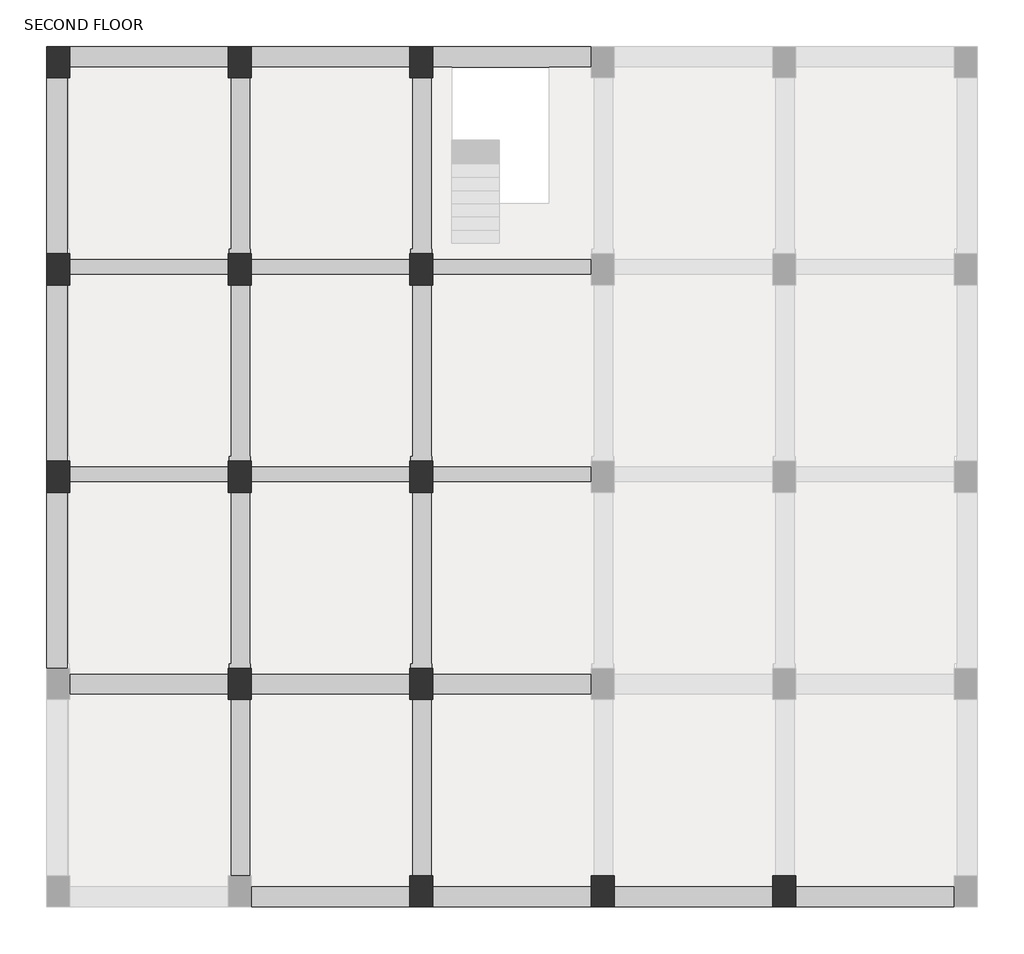
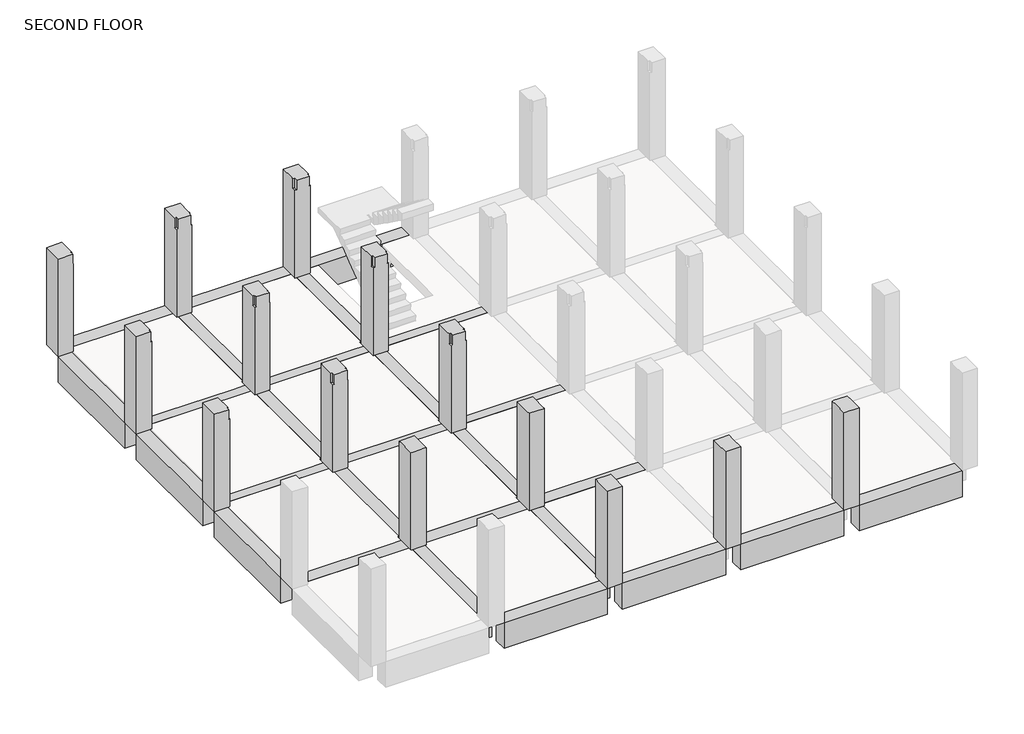
# One storey, part 2 of 3: 27 beams, 14 columns.
"""IFC4 building model written with IfcOpenShell, lengths in millimetres."""

from ifc_helpers import new_model, si_unit, frame, origin, place, context, project, spatial, polyline, outline, extrude, faceted_brep, element, save

model = new_model("IFC4")

# Units and contexts
model_context = context("Model", 3, world=origin())
ifc_project = project(units=[si_unit("LENGTHUNIT", "METRE", prefix="MILLI")], contexts=[model_context])

# Site, building, storey
site = spatial("IfcSite", under=ifc_project)
building = spatial("IfcBuilding", under=site)
storey = spatial("IfcBuildingStorey", under=building, Name="SECOND FLOOR", Elevation=6096.0)

# Beams
placement = place(None, origin())
element("IfcBeam", 1, ObjectType="M_Concrete-Rectangular Beam : 400 x 800mm", at=placement, inside=storey, context=model_context, shape_type="Brep", body=[
    faceted_brep([(4855.1115906, 3503.1212443, 6096.0), (4855.1115906, 3103.1212443, 6096.0), (7905.1115906, 3103.1212443, 6096.0), (7905.1115906, 3503.1212443, 6096.0), (4855.1115906, 3503.1212443, 5296.0), (4855.1115906, 3503.1212443, 5796.0), (7905.1115906, 3503.1212443, 5796.0), (7905.1115906, 3503.1212443, 5296.0), (4855.1115906, 3103.1212443, 5296.0), (7905.1115906, 3103.1212443, 5296.0)], [[[0, 1, 2, 3]], [[4, 5, 0, 3, 6, 7]], [[8, 4, 7, 9]], [[1, 8, 9, 2]], [[1, 0, 5, 4, 8]], [[3, 2, 9, 7, 6]]]),
])
element("IfcBeam", 2, ObjectType="M_Concrete-Rectangular Beam : 400 x 800mm", at=placement, inside=storey, context=model_context, shape_type="Brep", body=[
    faceted_brep([(1355.1115906, 3503.1212443, 6096.0), (1355.1115906, 3103.1212443, 6096.0), (4405.1115906, 3103.1212443, 6096.0), (4405.1115906, 3503.1212443, 6096.0), (1355.1115906, 3503.1212443, 5296.0), (1355.1115906, 3503.1212443, 5796.0), (4405.1115906, 3503.1212443, 5796.0), (4405.1115906, 3503.1212443, 5296.0), (1355.1115906, 3103.1212443, 5296.0), (4405.1115906, 3103.1212443, 5296.0)], [[[0, 1, 2, 3]], [[4, 5, 0, 3, 6, 7]], [[8, 4, 7, 9]], [[1, 8, 9, 2]], [[1, 0, 5, 4, 8]], [[3, 2, 9, 7, 6]]]),
])
element("IfcBeam", 3, ObjectType="M_Concrete-Rectangular Beam : 400 x 800mm", at=placement, inside=storey, context=model_context, shape_type="Brep", body=[
    faceted_brep([(-2144.8884094, 3503.1212443, 6096.0), (-2144.8884094, 3103.1212443, 6096.0), (905.1115906, 3103.1212443, 6096.0), (905.1115906, 3503.1212443, 6096.0), (-2144.8884094, 3503.1212443, 5296.0), (-2144.8884094, 3503.1212443, 5796.0), (905.1115906, 3503.1212443, 5796.0), (905.1115906, 3503.1212443, 5296.0), (-2144.8884094, 3103.1212443, 5296.0), (905.1115906, 3103.1212443, 5296.0)], [[[0, 1, 2, 3]], [[4, 5, 0, 3, 6, 7]], [[8, 4, 7, 9]], [[1, 8, 9, 2]], [[1, 0, 5, 4, 8]], [[3, 2, 9, 7, 6]]]),
])
element("IfcBeam", 4, ObjectType="M_Concrete-Rectangular Beam : 400 x 800mm", at=placement, inside=storey, context=model_context, shape_type="Brep", body=[
    faceted_brep([(-5644.8884094, 3503.1212443, 6096.0), (-5644.8884094, 3103.1212443, 6096.0), (-2594.8884094, 3103.1212443, 6096.0), (-2594.8884094, 3503.1212443, 6096.0), (-5644.8884094, 3503.1212443, 5296.0), (-5644.8884094, 3503.1212443, 5796.0), (-2594.8884094, 3503.1212443, 5796.0), (-2594.8884094, 3503.1212443, 5296.0), (-5644.8884094, 3103.1212443, 5296.0), (-2594.8884094, 3103.1212443, 5296.0)], [[[0, 1, 2, 3]], [[4, 5, 0, 3, 6, 7]], [[8, 4, 7, 9]], [[1, 8, 9, 2]], [[1, 0, 5, 4, 8]], [[3, 2, 9, 7, 6]]]),
])
element("IfcBeam", 5, ObjectType="M_Concrete-Rectangular Beam : 400 x 800mm", at=placement, inside=storey, context=model_context, shape_type="SweptSolid", body=[
    extrude(outline(polyline([(-9594.8884094, 11103.1212443), (-9194.8884094, 11103.1212443), (-9194.8884094, 7703.1212443), (-9594.8884094, 7703.1212443), (-9594.8884094, 11103.1212443)])), frame((0.0, 0.0, 5296.0), z_axis=(0.0, 0.0, 1.0), x_axis=(1.0, 0.0, 0.0)), (0.0, 0.0, 1.0), 800.0),
])
element("IfcBeam", 6, ObjectType="M_Concrete-Rectangular Beam : 400 x 800mm", at=placement, inside=storey, context=model_context, shape_type="SweptSolid", body=[
    extrude(outline(polyline([(-9594.8884094, 15103.1212443), (-9194.8884094, 15103.1212443), (-9194.8884094, 11703.1212443), (-9594.8884094, 11703.1212443), (-9594.8884094, 15103.1212443)])), frame((0.0, 0.0, 5296.0), z_axis=(0.0, 0.0, 1.0), x_axis=(1.0, 0.0, 0.0)), (0.0, 0.0, 1.0), 800.0),
])
element("IfcBeam", 7, ObjectType="M_Concrete-Rectangular Beam : 400 x 800mm", at=placement, inside=storey, context=model_context, shape_type="Brep", body=[
    faceted_brep([(-2594.8884094, 19303.1212443, 6096.0), (-2594.8884094, 19703.1212443, 6096.0), (-5644.8884094, 19703.1212443, 6096.0), (-5644.8884094, 19303.1212443, 6096.0), (-2594.8884094, 19303.1212443, 5296.0), (-2594.8884094, 19303.1212443, 5796.0), (-5644.8884094, 19303.1212443, 5796.0), (-5644.8884094, 19303.1212443, 5296.0), (-2594.8884094, 19703.1212443, 5296.0), (-5644.8884094, 19703.1212443, 5296.0)], [[[0, 1, 2, 3]], [[4, 5, 0, 3, 6, 7]], [[8, 4, 7, 9]], [[1, 8, 9, 2]], [[1, 0, 5, 4, 8]], [[3, 2, 9, 7, 6]]]),
])
element("IfcBeam", 8, ObjectType="M_Concrete-Rectangular Beam : 400 x 800mm", at=placement, inside=storey, context=model_context, shape_type="Brep", body=[
    faceted_brep([(-2144.8884094, 19703.1212443, 6096.0), (-2144.8884094, 19303.1212443, 6096.0), (-1784.8884094, 19303.1212443, 6096.0), (94.7115906, 19303.1212443, 6096.0), (905.1115906, 19303.1212443, 6096.0), (905.1115906, 19703.1212443, 6096.0), (-2144.8884094, 19303.1212443, 5796.0), (-2144.8884094, 19303.1212443, 5296.0), (905.1115906, 19303.1212443, 5296.0), (905.1115906, 19303.1212443, 5796.0), (-2144.8884094, 19703.1212443, 5296.0), (905.1115906, 19703.1212443, 5296.0)], [[[0, 1, 2, 3, 4, 5]], [[1, 6, 7, 8, 9, 4, 3, 2]], [[7, 10, 11, 8]], [[10, 0, 5, 11]], [[1, 0, 10, 7, 6]], [[5, 4, 9, 8, 11]]]),
])
element("IfcBeam", 9, ObjectType="M_Concrete-Rectangular Beam : 400 x 800mm", at=placement, inside=storey, context=model_context, shape_type="Brep", body=[
    faceted_brep([(-5669.8884094, 15703.1212443, 6096.0), (-5669.8884094, 15803.1212443, 6096.0), (-5669.8884094, 19103.1212443, 6096.0), (-6044.8884094, 19103.1212443, 6096.0), (-6044.8884094, 15803.1212443, 6096.0), (-6069.8884094, 15803.1212443, 6096.0), (-6069.8884094, 15703.1212443, 6096.0), (-6069.8884094, 19103.1212443, 5296.0), (-6069.8884094, 15703.1212443, 5296.0), (-6069.8884094, 15803.1212443, 5796.0), (-6069.8884094, 19103.1212443, 5796.0), (-5669.8884094, 19103.1212443, 5296.0), (-5669.8884094, 15703.1212443, 5296.0), (-6044.8884094, 19103.1212443, 5796.0), (-6044.8884094, 15803.1212443, 5796.0)], [[[0, 1, 2, 3, 4, 5, 6]], [[7, 8, 6, 5, 9, 10]], [[7, 11, 12, 8]], [[11, 2, 1, 0, 12]], [[11, 7, 10, 13, 3, 2]], [[0, 6, 8, 12]], [[9, 14, 13, 10]], [[14, 4, 3, 13]], [[4, 14, 9, 5]]]),
])
element("IfcBeam", 10, ObjectType="M_Concrete-Rectangular Beam : 400 x 800mm", at=placement, inside=storey, context=model_context, shape_type="Brep", body=[
    faceted_brep([(-5669.8884094, 11703.1212443, 6096.0), (-5669.8884094, 11803.1212443, 6096.0), (-5669.8884094, 15103.1212443, 6096.0), (-6044.8884094, 15103.1212443, 6096.0), (-6044.8884094, 11803.1212443, 6096.0), (-6069.8884094, 11803.1212443, 6096.0), (-6069.8884094, 11703.1212443, 6096.0), (-6069.8884094, 15103.1212443, 5296.0), (-6069.8884094, 11703.1212443, 5296.0), (-6069.8884094, 11803.1212443, 5796.0), (-6069.8884094, 15103.1212443, 5796.0), (-5669.8884094, 15103.1212443, 5296.0), (-5669.8884094, 11703.1212443, 5296.0), (-6044.8884094, 15103.1212443, 5796.0), (-6044.8884094, 11803.1212443, 5796.0)], [[[0, 1, 2, 3, 4, 5, 6]], [[7, 8, 6, 5, 9, 10]], [[7, 11, 12, 8]], [[11, 2, 1, 0, 12]], [[11, 7, 10, 13, 3, 2]], [[0, 6, 8, 12]], [[9, 14, 13, 10]], [[14, 4, 3, 13]], [[4, 14, 9, 5]]]),
])
element("IfcBeam", 11, ObjectType="M_Concrete-Rectangular Beam : 400 x 800mm", at=placement, inside=storey, context=model_context, shape_type="Brep", body=[
    faceted_brep([(-5669.8884094, 7703.1212443, 6096.0), (-5669.8884094, 7803.1212443, 6096.0), (-5669.8884094, 11103.1212443, 6096.0), (-6044.8884094, 11103.1212443, 6096.0), (-6044.8884094, 7803.1212443, 6096.0), (-6069.8884094, 7803.1212443, 6096.0), (-6069.8884094, 7703.1212443, 6096.0), (-6069.8884094, 11103.1212443, 5296.0), (-6069.8884094, 7703.1212443, 5296.0), (-6069.8884094, 7803.1212443, 5796.0), (-6069.8884094, 11103.1212443, 5796.0), (-5669.8884094, 11103.1212443, 5296.0), (-5669.8884094, 7703.1212443, 5296.0), (-6044.8884094, 11103.1212443, 5796.0), (-6044.8884094, 7803.1212443, 5796.0)], [[[0, 1, 2, 3, 4, 5, 6]], [[7, 8, 6, 5, 9, 10]], [[8, 7, 11, 12]], [[2, 1, 0, 12, 11]], [[2, 11, 7, 10, 13, 3]], [[0, 6, 8, 12]], [[9, 14, 13, 10]], [[14, 4, 3, 13]], [[4, 14, 9, 5]]]),
])
element("IfcBeam", 12, ObjectType="M_Concrete-Rectangular Beam : 400 x 800mm", at=placement, inside=storey, context=model_context, shape_type="Brep", body=[
    faceted_brep([(-5669.8884094, 3703.1212443, 6096.0), (-5669.8884094, 7103.1212443, 6096.0), (-6044.8884094, 7103.1212443, 6096.0), (-6044.8884094, 3703.1212443, 6096.0), (-6069.8884094, 7103.1212443, 5296.0), (-6069.8884094, 3703.1212443, 5296.0), (-6069.8884094, 3703.1212443, 5796.0), (-6069.8884094, 7103.1212443, 5796.0), (-5669.8884094, 7103.1212443, 5296.0), (-5669.8884094, 3703.1212443, 5296.0), (-5669.8884094, 7103.1212443, 5796.0), (-5669.8884094, 3703.1212443, 5796.0), (-6044.8884094, 7103.1212443, 5796.0), (-6044.8884094, 3703.1212443, 5796.0)], [[[0, 1, 2, 3]], [[4, 5, 6, 7]], [[4, 8, 9, 5]], [[8, 10, 1, 0, 11, 9]], [[8, 4, 7, 12, 2, 1, 10]], [[5, 9, 11, 0, 3, 13, 6]], [[13, 12, 7, 6]], [[12, 13, 3, 2]]]),
])
element("IfcBeam", 13, ObjectType="M_Concrete-Rectangular Beam : 400 x 800mm", at=placement, inside=storey, context=model_context, shape_type="Brep", body=[
    faceted_brep([(-2169.8884094, 15703.1212443, 6096.0), (-2169.8884094, 15803.1212443, 6096.0), (-2169.8884094, 19103.1212443, 6096.0), (-2544.8884094, 19103.1212443, 6096.0), (-2544.8884094, 15803.1212443, 6096.0), (-2569.8884094, 15803.1212443, 6096.0), (-2569.8884094, 15703.1212443, 6096.0), (-2569.8884094, 19103.1212443, 5296.0), (-2569.8884094, 15703.1212443, 5296.0), (-2569.8884094, 15803.1212443, 5796.0), (-2569.8884094, 19103.1212443, 5796.0), (-2169.8884094, 19103.1212443, 5296.0), (-2169.8884094, 15703.1212443, 5296.0), (-2544.8884094, 19103.1212443, 5796.0), (-2544.8884094, 15803.1212443, 5796.0)], [[[0, 1, 2, 3, 4, 5, 6]], [[7, 8, 6, 5, 9, 10]], [[7, 11, 12, 8]], [[11, 2, 1, 0, 12]], [[11, 7, 10, 13, 3, 2]], [[0, 6, 8, 12]], [[9, 14, 13, 10]], [[14, 4, 3, 13]], [[4, 14, 9, 5]]]),
])
element("IfcBeam", 14, ObjectType="M_Concrete-Rectangular Beam : 400 x 800mm", at=placement, inside=storey, context=model_context, shape_type="Brep", body=[
    faceted_brep([(-2169.8884094, 11703.1212443, 6096.0), (-2169.8884094, 11803.1212443, 6096.0), (-2169.8884094, 15103.1212443, 6096.0), (-2544.8884094, 15103.1212443, 6096.0), (-2544.8884094, 11803.1212443, 6096.0), (-2569.8884094, 11803.1212443, 6096.0), (-2569.8884094, 11703.1212443, 6096.0), (-2569.8884094, 15103.1212443, 5296.0), (-2569.8884094, 11703.1212443, 5296.0), (-2569.8884094, 11803.1212443, 5796.0), (-2569.8884094, 15103.1212443, 5796.0), (-2169.8884094, 15103.1212443, 5296.0), (-2169.8884094, 11703.1212443, 5296.0), (-2544.8884094, 15103.1212443, 5796.0), (-2544.8884094, 11803.1212443, 5796.0)], [[[0, 1, 2, 3, 4, 5, 6]], [[7, 8, 6, 5, 9, 10]], [[8, 7, 11, 12]], [[2, 1, 0, 12, 11]], [[2, 11, 7, 10, 13, 3]], [[0, 6, 8, 12]], [[9, 14, 13, 10]], [[14, 4, 3, 13]], [[4, 14, 9, 5]]]),
])
element("IfcBeam", 15, ObjectType="M_Concrete-Rectangular Beam : 400 x 800mm", at=placement, inside=storey, context=model_context, shape_type="Brep", body=[
    faceted_brep([(-2169.8884094, 7703.1212443, 6096.0), (-2169.8884094, 7803.1212443, 6096.0), (-2169.8884094, 11103.1212443, 6096.0), (-2544.8884094, 11103.1212443, 6096.0), (-2544.8884094, 7803.1212443, 6096.0), (-2569.8884094, 7803.1212443, 6096.0), (-2569.8884094, 7703.1212443, 6096.0), (-2569.8884094, 11103.1212443, 5296.0), (-2569.8884094, 7703.1212443, 5296.0), (-2569.8884094, 7803.1212443, 5796.0), (-2569.8884094, 11103.1212443, 5796.0), (-2169.8884094, 11103.1212443, 5296.0), (-2169.8884094, 7703.1212443, 5296.0), (-2544.8884094, 11103.1212443, 5796.0), (-2544.8884094, 7803.1212443, 5796.0)], [[[0, 1, 2, 3, 4, 5, 6]], [[7, 8, 6, 5, 9, 10]], [[7, 11, 12, 8]], [[11, 2, 1, 0, 12]], [[2, 11, 7, 10, 13, 3]], [[0, 6, 8, 12]], [[9, 14, 13, 10]], [[14, 4, 3, 13]], [[4, 14, 9, 5]]]),
])
element("IfcBeam", 16, ObjectType="M_Concrete-Rectangular Beam : 400 x 800mm", at=placement, inside=storey, context=model_context, shape_type="Brep", body=[
    faceted_brep([(-2169.8884094, 3703.1212443, 6096.0), (-2169.8884094, 7103.1212443, 6096.0), (-2544.8884094, 7103.1212443, 6096.0), (-2544.8884094, 3703.1212443, 6096.0), (-2569.8884094, 7103.1212443, 5296.0), (-2569.8884094, 3703.1212443, 5296.0), (-2569.8884094, 3703.1212443, 5796.0), (-2569.8884094, 7103.1212443, 5796.0), (-2169.8884094, 7103.1212443, 5296.0), (-2169.8884094, 3703.1212443, 5296.0), (-2169.8884094, 7103.1212443, 5796.0), (-2169.8884094, 3703.1212443, 5796.0), (-2544.8884094, 7103.1212443, 5796.0), (-2544.8884094, 3703.1212443, 5796.0)], [[[0, 1, 2, 3]], [[4, 5, 6, 7]], [[4, 8, 9, 5]], [[8, 10, 1, 0, 11, 9]], [[8, 4, 7, 12, 2, 1, 10]], [[5, 9, 11, 0, 3, 13, 6]], [[13, 12, 7, 6]], [[12, 13, 3, 2]]]),
])
element("IfcBeam", 17, ObjectType="M_Concrete-Rectangular Beam : 400 x 800mm", at=placement, inside=storey, context=model_context, shape_type="Brep", body=[
    faceted_brep([(-6094.8884094, 15603.1212443, 6096.0), (-9144.8884094, 15603.1212443, 6096.0), (-9144.8884094, 15303.1212443, 6096.0), (-6094.8884094, 15303.1212443, 6096.0), (-9144.8884094, 15203.1212443, 5296.0), (-6094.8884094, 15203.1212443, 5296.0), (-6094.8884094, 15203.1212443, 5796.0), (-9144.8884094, 15203.1212443, 5796.0), (-9144.8884094, 15603.1212443, 5296.0), (-6094.8884094, 15603.1212443, 5296.0), (-9144.8884094, 15603.1212443, 5796.0), (-6094.8884094, 15603.1212443, 5796.0), (-9144.8884094, 15303.1212443, 5796.0), (-6094.8884094, 15303.1212443, 5796.0)], [[[0, 1, 2, 3]], [[4, 5, 6, 7]], [[4, 8, 9, 5]], [[8, 10, 1, 0, 11, 9]], [[8, 4, 7, 12, 2, 1, 10]], [[5, 9, 11, 0, 3, 13, 6]], [[13, 12, 7, 6]], [[12, 13, 3, 2]]]),
])
element("IfcBeam", 18, ObjectType="M_Concrete-Rectangular Beam : 400 x 800mm", at=placement, inside=storey, context=model_context, shape_type="Brep", body=[
    faceted_brep([(-2594.8884094, 15603.1212443, 6096.0), (-5644.8884094, 15603.1212443, 6096.0), (-5644.8884094, 15303.1212443, 6096.0), (-2594.8884094, 15303.1212443, 6096.0), (-5644.8884094, 15203.1212443, 5296.0), (-2594.8884094, 15203.1212443, 5296.0), (-2594.8884094, 15203.1212443, 5796.0), (-5644.8884094, 15203.1212443, 5796.0), (-5644.8884094, 15603.1212443, 5296.0), (-2594.8884094, 15603.1212443, 5296.0), (-5644.8884094, 15603.1212443, 5796.0), (-2594.8884094, 15603.1212443, 5796.0), (-5644.8884094, 15303.1212443, 5796.0), (-2594.8884094, 15303.1212443, 5796.0)], [[[0, 1, 2, 3]], [[4, 5, 6, 7]], [[4, 8, 9, 5]], [[8, 10, 1, 0, 11, 9]], [[8, 4, 7, 12, 2, 1, 10]], [[5, 9, 11, 0, 3, 13, 6]], [[13, 12, 7, 6]], [[12, 13, 3, 2]]]),
])
element("IfcBeam", 19, ObjectType="M_Concrete-Rectangular Beam : 400 x 800mm", at=placement, inside=storey, context=model_context, shape_type="Brep", body=[
    faceted_brep([(905.1115906, 15603.1212443, 6096.0), (-2144.8884094, 15603.1212443, 6096.0), (-2144.8884094, 15303.1212443, 6096.0), (905.1115906, 15303.1212443, 6096.0), (-2144.8884094, 15603.1212443, 5296.0), (-2144.8884094, 15603.1212443, 5796.0), (905.1115906, 15603.1212443, 5796.0), (905.1115906, 15603.1212443, 5296.0), (-2144.8884094, 15203.1212443, 5296.0), (905.1115906, 15203.1212443, 5296.0), (905.1115906, 15203.1212443, 5796.0), (-2144.8884094, 15203.1212443, 5796.0), (-2144.8884094, 15303.1212443, 5796.0), (905.1115906, 15303.1212443, 5796.0)], [[[0, 1, 2, 3]], [[4, 5, 1, 0, 6, 7]], [[8, 4, 7, 9]], [[8, 9, 10, 11]], [[1, 5, 4, 8, 11, 12, 2]], [[7, 6, 0, 3, 13, 10, 9]], [[13, 12, 11, 10]], [[12, 13, 3, 2]]]),
])
element("IfcBeam", 20, ObjectType="M_Concrete-Rectangular Beam : 400 x 800mm", at=placement, inside=storey, context=model_context, shape_type="Brep", body=[
    faceted_brep([(905.1115906, 11603.1212443, 6096.0), (-2144.8884094, 11603.1212443, 6096.0), (-2144.8884094, 11303.1212443, 6096.0), (905.1115906, 11303.1212443, 6096.0), (-2144.8884094, 11603.1212443, 5296.0), (-2144.8884094, 11603.1212443, 5796.0), (905.1115906, 11603.1212443, 5796.0), (905.1115906, 11603.1212443, 5296.0), (-2144.8884094, 11203.1212443, 5296.0), (905.1115906, 11203.1212443, 5296.0), (905.1115906, 11203.1212443, 5796.0), (-2144.8884094, 11203.1212443, 5796.0), (-2144.8884094, 11303.1212443, 5796.0), (905.1115906, 11303.1212443, 5796.0)], [[[0, 1, 2, 3]], [[4, 5, 1, 0, 6, 7]], [[8, 4, 7, 9]], [[8, 9, 10, 11]], [[1, 5, 4, 8, 11, 12, 2]], [[7, 6, 0, 3, 13, 10, 9]], [[13, 12, 11, 10]], [[12, 13, 3, 2]]]),
])
element("IfcBeam", 21, ObjectType="M_Concrete-Rectangular Beam : 400 x 800mm", at=placement, inside=storey, context=model_context, shape_type="Brep", body=[
    faceted_brep([(-2594.8884094, 11603.1212443, 6096.0), (-5644.8884094, 11603.1212443, 6096.0), (-5644.8884094, 11303.1212443, 6096.0), (-2594.8884094, 11303.1212443, 6096.0), (-5644.8884094, 11603.1212443, 5296.0), (-5644.8884094, 11603.1212443, 5796.0), (-2594.8884094, 11603.1212443, 5796.0), (-2594.8884094, 11603.1212443, 5296.0), (-5644.8884094, 11203.1212443, 5296.0), (-2594.8884094, 11203.1212443, 5296.0), (-2594.8884094, 11203.1212443, 5796.0), (-5644.8884094, 11203.1212443, 5796.0), (-5644.8884094, 11303.1212443, 5796.0), (-2594.8884094, 11303.1212443, 5796.0)], [[[0, 1, 2, 3]], [[4, 5, 1, 0, 6, 7]], [[8, 4, 7, 9]], [[8, 9, 10, 11]], [[1, 5, 4, 8, 11, 12, 2]], [[7, 6, 0, 3, 13, 10, 9]], [[13, 12, 11, 10]], [[12, 13, 3, 2]]]),
])
element("IfcBeam", 22, ObjectType="M_Concrete-Rectangular Beam : 400 x 800mm", at=placement, inside=storey, context=model_context, shape_type="Brep", body=[
    faceted_brep([(-6094.8884094, 11603.1212443, 6096.0), (-9144.8884094, 11603.1212443, 6096.0), (-9144.8884094, 11303.1212443, 6096.0), (-6094.8884094, 11303.1212443, 6096.0), (-9144.8884094, 11603.1212443, 5296.0), (-9144.8884094, 11603.1212443, 5796.0), (-6094.8884094, 11603.1212443, 5796.0), (-6094.8884094, 11603.1212443, 5296.0), (-9144.8884094, 11203.1212443, 5296.0), (-6094.8884094, 11203.1212443, 5296.0), (-6094.8884094, 11203.1212443, 5796.0), (-9144.8884094, 11203.1212443, 5796.0), (-9144.8884094, 11303.1212443, 5796.0), (-6094.8884094, 11303.1212443, 5796.0)], [[[0, 1, 2, 3]], [[4, 5, 1, 0, 6, 7]], [[8, 4, 7, 9]], [[8, 9, 10, 11]], [[1, 5, 4, 8, 11, 12, 2]], [[7, 6, 0, 3, 13, 10, 9]], [[13, 12, 11, 10]], [[12, 13, 3, 2]]]),
])
element("IfcBeam", 23, ObjectType="M_Concrete-Rectangular Beam : 400 x 800mm", at=placement, inside=storey, context=model_context, shape_type="Brep", body=[
    faceted_brep([(-9144.8884094, 7603.1212443, 6096.0), (-9144.8884094, 7203.1212443, 6096.0), (-6094.8884094, 7203.1212443, 6096.0), (-6094.8884094, 7603.1212443, 6096.0), (-9144.8884094, 7203.1212443, 5796.0), (-9144.8884094, 7203.1212443, 5296.0), (-6094.8884094, 7203.1212443, 5296.0), (-6094.8884094, 7203.1212443, 5796.0), (-9144.8884094, 7603.1212443, 5296.0), (-6094.8884094, 7603.1212443, 5296.0), (-9144.8884094, 7603.1212443, 5796.0), (-6094.8884094, 7603.1212443, 5796.0)], [[[0, 1, 2, 3]], [[1, 4, 5, 6, 7, 2]], [[5, 8, 9, 6]], [[8, 10, 0, 3, 11, 9]], [[1, 0, 10, 8, 5, 4]], [[3, 2, 7, 6, 9, 11]]]),
])
element("IfcBeam", 24, ObjectType="M_Concrete-Rectangular Beam : 400 x 800mm", at=placement, inside=storey, context=model_context, shape_type="Brep", body=[
    faceted_brep([(-5644.8884094, 7603.1212443, 6096.0), (-5644.8884094, 7203.1212443, 6096.0), (-2594.8884094, 7203.1212443, 6096.0), (-2594.8884094, 7603.1212443, 6096.0), (-5644.8884094, 7203.1212443, 5796.0), (-5644.8884094, 7203.1212443, 5296.0), (-2594.8884094, 7203.1212443, 5296.0), (-2594.8884094, 7203.1212443, 5796.0), (-5644.8884094, 7603.1212443, 5296.0), (-2594.8884094, 7603.1212443, 5296.0), (-5644.8884094, 7603.1212443, 5796.0), (-2594.8884094, 7603.1212443, 5796.0)], [[[0, 1, 2, 3]], [[1, 4, 5, 6, 7, 2]], [[5, 8, 9, 6]], [[8, 10, 0, 3, 11, 9]], [[1, 0, 10, 8, 5, 4]], [[3, 2, 7, 6, 9, 11]]]),
])
element("IfcBeam", 25, ObjectType="M_Concrete-Rectangular Beam : 400 x 800mm", at=placement, inside=storey, context=model_context, shape_type="Brep", body=[
    faceted_brep([(-2144.8884094, 7603.1212443, 6096.0), (-2144.8884094, 7203.1212443, 6096.0), (905.1115906, 7203.1212443, 6096.0), (905.1115906, 7603.1212443, 6096.0), (-2144.8884094, 7203.1212443, 5796.0), (-2144.8884094, 7203.1212443, 5296.0), (905.1115906, 7203.1212443, 5296.0), (905.1115906, 7203.1212443, 5796.0), (-2144.8884094, 7603.1212443, 5296.0), (905.1115906, 7603.1212443, 5296.0), (-2144.8884094, 7603.1212443, 5796.0), (905.1115906, 7603.1212443, 5796.0)], [[[0, 1, 2, 3]], [[1, 4, 5, 6, 7, 2]], [[5, 8, 9, 6]], [[8, 10, 0, 3, 11, 9]], [[1, 0, 10, 8, 5, 4]], [[3, 2, 7, 6, 9, 11]]]),
])
element("IfcBeam", 26, ObjectType="M_Concrete-Rectangular Beam : 400 x 800mm", at=placement, inside=storey, context=model_context, shape_type="SweptSolid", body=[
    extrude(outline(polyline([(-9594.8884094, 19103.1212443), (-9194.8884094, 19103.1212443), (-9194.8884094, 15703.1212443), (-9594.8884094, 15703.1212443), (-9594.8884094, 19103.1212443)])), frame((0.0, 0.0, 5296.0), z_axis=(0.0, 0.0, 1.0), x_axis=(1.0, 0.0, 0.0)), (0.0, 0.0, 1.0), 800.0),
])
element("IfcBeam", 27, ObjectType="M_Concrete-Rectangular Beam : 400 x 800mm", at=placement, inside=storey, context=model_context, shape_type="Brep", body=[
    faceted_brep([(-6094.8884094, 19303.1212443, 6096.0), (-6094.8884094, 19703.1212443, 6096.0), (-9144.8884094, 19703.1212443, 6096.0), (-9144.8884094, 19303.1212443, 6096.0), (-6094.8884094, 19303.1212443, 5296.0), (-6094.8884094, 19303.1212443, 5796.0), (-9144.8884094, 19303.1212443, 5796.0), (-9144.8884094, 19303.1212443, 5296.0), (-6094.8884094, 19703.1212443, 5296.0), (-9144.8884094, 19703.1212443, 5296.0)], [[[0, 1, 2, 3]], [[4, 5, 0, 3, 6, 7]], [[8, 4, 7, 9]], [[1, 8, 9, 2]], [[2, 9, 7, 6, 3]], [[1, 0, 5, 4, 8]]]),
])

# Columns
element("IfcColumn", 28, ObjectType="M_Concrete-Rectangular-Column : 450 x 600mm", at=placement, inside=storey, context=model_context, shape_type="Brep", body=[
    faceted_brep([(-9144.8884094, 19703.1212443, 6096.0), (-9144.8884094, 19103.1212443, 6096.0), (-9594.8884094, 19103.1212443, 6096.0), (-9594.8884094, 19703.1212443, 6096.0), (-9144.8884094, 19703.1212443, 9144.0), (-9144.8884094, 19303.1212443, 9144.0), (-9144.8884094, 19203.1212443, 9144.0), (-9144.8884094, 19203.1212443, 8844.0), (-9144.8884094, 19103.1212443, 8844.0), (-9169.8884094, 19103.1212443, 8844.0), (-9169.8884094, 19103.1212443, 9144.0), (-9594.8884094, 19103.1212443, 9144.0), (-9594.8884094, 19703.1212443, 9144.0), (-9169.8884094, 19203.1212443, 9144.0), (-9169.8884094, 19203.1212443, 8844.0)], [[[0, 1, 2, 3]], [[1, 0, 4, 5, 6, 7, 8]], [[2, 1, 8, 9, 10, 11]], [[3, 2, 11, 12]], [[0, 3, 12, 4]], [[12, 11, 10, 13, 6, 5, 4]], [[7, 14, 9, 8]], [[14, 13, 10, 9]], [[14, 7, 6, 13]]]),
])
element("IfcColumn", 29, ObjectType="M_Concrete-Rectangular-Column : 450 x 600mm", at=placement, inside=storey, context=model_context, shape_type="Brep", body=[
    faceted_brep([(-5644.8884094, 19703.1212443, 6096.0), (-5644.8884094, 19103.1212443, 6096.0), (-6094.8884094, 19103.1212443, 6096.0), (-6094.8884094, 19703.1212443, 6096.0), (-5644.8884094, 19703.1212443, 9144.0), (-5644.8884094, 19303.1212443, 9144.0), (-5644.8884094, 19203.1212443, 9144.0), (-5644.8884094, 19203.1212443, 8844.0), (-5644.8884094, 19103.1212443, 8844.0), (-5669.8884094, 19103.1212443, 8844.0), (-5669.8884094, 19103.1212443, 9144.0), (-6044.8884094, 19103.1212443, 9144.0), (-6044.8884094, 19103.1212443, 8844.0), (-6094.8884094, 19103.1212443, 8844.0), (-6094.8884094, 19203.1212443, 8844.0), (-6094.8884094, 19203.1212443, 9144.0), (-6094.8884094, 19303.1212443, 9144.0), (-6094.8884094, 19703.1212443, 9144.0), (-6044.8884094, 19203.1212443, 9144.0), (-5669.8884094, 19203.1212443, 9144.0), (-5669.8884094, 19203.1212443, 8844.0), (-6044.8884094, 19203.1212443, 8844.0)], [[[0, 1, 2, 3]], [[1, 0, 4, 5, 6, 7, 8]], [[2, 1, 8, 9, 10, 11, 12, 13]], [[3, 2, 13, 14, 15, 16, 17]], [[0, 3, 17, 4]], [[4, 17, 16, 15, 18, 11, 10, 19, 6, 5]], [[7, 20, 9, 8]], [[20, 19, 10, 9]], [[20, 7, 6, 19]], [[21, 14, 13, 12]], [[18, 21, 12, 11]], [[14, 21, 18, 15]]]),
])
element("IfcColumn", 30, ObjectType="M_Concrete-Rectangular-Column : 450 x 600mm", at=placement, inside=storey, context=model_context, shape_type="Brep", body=[
    faceted_brep([(-2144.8884094, 19703.1212443, 6096.0), (-2144.8884094, 19103.1212443, 6096.0), (-2594.8884094, 19103.1212443, 6096.0), (-2594.8884094, 19703.1212443, 6096.0), (-2144.8884094, 19703.1212443, 9144.0), (-2144.8884094, 19303.1212443, 9144.0), (-2144.8884094, 19203.1212443, 9144.0), (-2144.8884094, 19203.1212443, 8844.0), (-2144.8884094, 19103.1212443, 8844.0), (-2169.8884094, 19103.1212443, 8844.0), (-2169.8884094, 19103.1212443, 9144.0), (-2544.8884094, 19103.1212443, 9144.0), (-2544.8884094, 19103.1212443, 8844.0), (-2594.8884094, 19103.1212443, 8844.0), (-2594.8884094, 19203.1212443, 8844.0), (-2594.8884094, 19203.1212443, 9144.0), (-2594.8884094, 19303.1212443, 9144.0), (-2594.8884094, 19703.1212443, 9144.0), (-2544.8884094, 19203.1212443, 9144.0), (-2169.8884094, 19203.1212443, 9144.0), (-2169.8884094, 19203.1212443, 8844.0), (-2544.8884094, 19203.1212443, 8844.0)], [[[0, 1, 2, 3]], [[1, 0, 4, 5, 6, 7, 8]], [[2, 1, 8, 9, 10, 11, 12, 13]], [[3, 2, 13, 14, 15, 16, 17]], [[0, 3, 17, 4]], [[4, 17, 16, 15, 18, 11, 10, 19, 6, 5]], [[7, 20, 9, 8]], [[20, 19, 10, 9]], [[20, 7, 6, 19]], [[21, 14, 13, 12]], [[18, 21, 12, 11]], [[14, 21, 18, 15]]]),
])
element("IfcColumn", 31, ObjectType="M_Concrete-Rectangular-Column : 450 x 600mm", at=placement, inside=storey, context=model_context, shape_type="Brep", body=[
    faceted_brep([(-9144.8884094, 15703.1212443, 6096.0), (-9144.8884094, 15103.1212443, 6096.0), (-9594.8884094, 15103.1212443, 6096.0), (-9594.8884094, 15703.1212443, 6096.0), (-9144.8884094, 15703.1212443, 8844.0), (-9144.8884094, 15703.1212443, 9144.0), (-9144.8884094, 15603.1212443, 9144.0), (-9144.8884094, 15303.1212443, 9144.0), (-9144.8884094, 15203.1212443, 9144.0), (-9144.8884094, 15203.1212443, 8844.0), (-9144.8884094, 15103.1212443, 8844.0), (-9169.8884094, 15103.1212443, 8844.0), (-9169.8884094, 15103.1212443, 9144.0), (-9594.8884094, 15103.1212443, 9144.0), (-9594.8884094, 15703.1212443, 9144.0), (-9169.8884094, 15203.1212443, 9144.0), (-9169.8884094, 15203.1212443, 8844.0)], [[[0, 1, 2, 3]], [[1, 0, 4, 5, 6, 7, 8, 9, 10]], [[2, 1, 10, 11, 12, 13]], [[3, 2, 13, 14]], [[0, 3, 14, 5, 4]], [[14, 13, 12, 15, 8, 7, 6, 5]], [[9, 16, 11, 10]], [[16, 15, 12, 11]], [[16, 9, 8, 15]]]),
])
element("IfcColumn", 32, ObjectType="M_Concrete-Rectangular-Column : 450 x 600mm", at=placement, inside=storey, context=model_context, shape_type="Brep", body=[
    faceted_brep([(-5644.8884094, 15703.1212443, 6096.0), (-5644.8884094, 15103.1212443, 6096.0), (-6094.8884094, 15103.1212443, 6096.0), (-6094.8884094, 15703.1212443, 6096.0), (-5644.8884094, 15703.1212443, 8844.0), (-5644.8884094, 15703.1212443, 9144.0), (-5644.8884094, 15603.1212443, 9144.0), (-5644.8884094, 15303.1212443, 9144.0), (-5644.8884094, 15203.1212443, 9144.0), (-5644.8884094, 15203.1212443, 8844.0), (-5644.8884094, 15103.1212443, 8844.0), (-5669.8884094, 15103.1212443, 8844.0), (-5669.8884094, 15103.1212443, 9144.0), (-6044.8884094, 15103.1212443, 9144.0), (-6044.8884094, 15103.1212443, 8844.0), (-6094.8884094, 15103.1212443, 8844.0), (-6094.8884094, 15203.1212443, 8844.0), (-6094.8884094, 15203.1212443, 9144.0), (-6094.8884094, 15303.1212443, 9144.0), (-6094.8884094, 15603.1212443, 9144.0), (-6094.8884094, 15703.1212443, 9144.0), (-6094.8884094, 15703.1212443, 8844.0), (-6044.8884094, 15203.1212443, 9144.0), (-5669.8884094, 15203.1212443, 9144.0), (-6044.8884094, 15203.1212443, 8844.0), (-5669.8884094, 15203.1212443, 8844.0)], [[[0, 1, 2, 3]], [[1, 0, 4, 5, 6, 7, 8, 9, 10]], [[2, 1, 10, 11, 12, 13, 14, 15]], [[3, 2, 15, 16, 17, 18, 19, 20, 21]], [[0, 3, 21, 20, 5, 4]], [[5, 20, 19, 18, 17, 22, 13, 12, 23, 8, 7, 6]], [[24, 16, 15, 14]], [[22, 24, 14, 13]], [[16, 24, 22, 17]], [[9, 25, 11, 10]], [[25, 23, 12, 11]], [[25, 9, 8, 23]]]),
])
element("IfcColumn", 33, ObjectType="M_Concrete-Rectangular-Column : 450 x 600mm", at=placement, inside=storey, context=model_context, shape_type="Brep", body=[
    faceted_brep([(-2144.8884094, 15703.1212443, 6096.0), (-2144.8884094, 15103.1212443, 6096.0), (-2594.8884094, 15103.1212443, 6096.0), (-2594.8884094, 15703.1212443, 6096.0), (-2144.8884094, 15703.1212443, 8844.0), (-2144.8884094, 15703.1212443, 9144.0), (-2144.8884094, 15603.1212443, 9144.0), (-2144.8884094, 15303.1212443, 9144.0), (-2144.8884094, 15203.1212443, 9144.0), (-2144.8884094, 15203.1212443, 8844.0), (-2144.8884094, 15103.1212443, 8844.0), (-2169.8884094, 15103.1212443, 8844.0), (-2169.8884094, 15103.1212443, 9144.0), (-2544.8884094, 15103.1212443, 9144.0), (-2544.8884094, 15103.1212443, 8844.0), (-2594.8884094, 15103.1212443, 8844.0), (-2594.8884094, 15203.1212443, 8844.0), (-2594.8884094, 15203.1212443, 9144.0), (-2594.8884094, 15303.1212443, 9144.0), (-2594.8884094, 15603.1212443, 9144.0), (-2594.8884094, 15703.1212443, 9144.0), (-2594.8884094, 15703.1212443, 8844.0), (-2544.8884094, 15203.1212443, 9144.0), (-2169.8884094, 15203.1212443, 9144.0), (-2169.8884094, 15203.1212443, 8844.0), (-2544.8884094, 15203.1212443, 8844.0)], [[[0, 1, 2, 3]], [[1, 0, 4, 5, 6, 7, 8, 9, 10]], [[2, 1, 10, 11, 12, 13, 14, 15]], [[3, 2, 15, 16, 17, 18, 19, 20, 21]], [[0, 3, 21, 20, 5, 4]], [[5, 20, 19, 18, 17, 22, 13, 12, 23, 8, 7, 6]], [[9, 24, 11, 10]], [[24, 23, 12, 11]], [[24, 9, 8, 23]], [[25, 16, 15, 14]], [[22, 25, 14, 13]], [[16, 25, 22, 17]]]),
])
element("IfcColumn", 34, ObjectType="M_Concrete-Rectangular-Column : 450 x 600mm", at=placement, inside=storey, context=model_context, shape_type="Brep", body=[
    faceted_brep([(-9144.8884094, 11703.1212443, 6096.0), (-9144.8884094, 11103.1212443, 6096.0), (-9594.8884094, 11103.1212443, 6096.0), (-9594.8884094, 11703.1212443, 6096.0), (-9144.8884094, 11703.1212443, 8844.0), (-9144.8884094, 11703.1212443, 9144.0), (-9144.8884094, 11603.1212443, 9144.0), (-9144.8884094, 11303.1212443, 9144.0), (-9144.8884094, 11203.1212443, 9144.0), (-9144.8884094, 11203.1212443, 8844.0), (-9144.8884094, 11103.1212443, 8844.0), (-9169.8884094, 11103.1212443, 8844.0), (-9169.8884094, 11103.1212443, 9144.0), (-9594.8884094, 11103.1212443, 9144.0), (-9594.8884094, 11703.1212443, 9144.0), (-9169.8884094, 11203.1212443, 9144.0), (-9169.8884094, 11203.1212443, 8844.0)], [[[0, 1, 2, 3]], [[1, 0, 4, 5, 6, 7, 8, 9, 10]], [[2, 1, 10, 11, 12, 13]], [[3, 2, 13, 14]], [[0, 3, 14, 5, 4]], [[14, 13, 12, 15, 8, 7, 6, 5]], [[9, 16, 11, 10]], [[16, 15, 12, 11]], [[16, 9, 8, 15]]]),
])
element("IfcColumn", 35, ObjectType="M_Concrete-Rectangular-Column : 450 x 600mm", at=placement, inside=storey, context=model_context, shape_type="Brep", body=[
    faceted_brep([(-5644.8884094, 11703.1212443, 6096.0), (-5644.8884094, 11103.1212443, 6096.0), (-6094.8884094, 11103.1212443, 6096.0), (-6094.8884094, 11703.1212443, 6096.0), (-5644.8884094, 11703.1212443, 8844.0), (-5644.8884094, 11703.1212443, 9144.0), (-5644.8884094, 11603.1212443, 9144.0), (-5644.8884094, 11303.1212443, 9144.0), (-5644.8884094, 11203.1212443, 9144.0), (-5644.8884094, 11203.1212443, 8844.0), (-5644.8884094, 11103.1212443, 8844.0), (-5669.8884094, 11103.1212443, 8844.0), (-5669.8884094, 11103.1212443, 9144.0), (-6044.8884094, 11103.1212443, 9144.0), (-6044.8884094, 11103.1212443, 8844.0), (-6094.8884094, 11103.1212443, 8844.0), (-6094.8884094, 11203.1212443, 8844.0), (-6094.8884094, 11203.1212443, 9144.0), (-6094.8884094, 11303.1212443, 9144.0), (-6094.8884094, 11603.1212443, 9144.0), (-6094.8884094, 11703.1212443, 9144.0), (-6094.8884094, 11703.1212443, 8844.0), (-6044.8884094, 11203.1212443, 9144.0), (-5669.8884094, 11203.1212443, 9144.0), (-5669.8884094, 11203.1212443, 8844.0), (-6044.8884094, 11203.1212443, 8844.0)], [[[0, 1, 2, 3]], [[1, 0, 4, 5, 6, 7, 8, 9, 10]], [[2, 1, 10, 11, 12, 13, 14, 15]], [[3, 2, 15, 16, 17, 18, 19, 20, 21]], [[0, 3, 21, 20, 5, 4]], [[5, 20, 19, 18, 17, 22, 13, 12, 23, 8, 7, 6]], [[9, 24, 11, 10]], [[24, 23, 12, 11]], [[24, 9, 8, 23]], [[25, 16, 15, 14]], [[22, 25, 14, 13]], [[16, 25, 22, 17]]]),
])
element("IfcColumn", 36, ObjectType="M_Concrete-Rectangular-Column : 450 x 600mm", at=placement, inside=storey, context=model_context, shape_type="Brep", body=[
    faceted_brep([(-2144.8884094, 11703.1212443, 6096.0), (-2144.8884094, 11103.1212443, 6096.0), (-2594.8884094, 11103.1212443, 6096.0), (-2594.8884094, 11703.1212443, 6096.0), (-2144.8884094, 11703.1212443, 8844.0), (-2144.8884094, 11703.1212443, 9144.0), (-2144.8884094, 11603.1212443, 9144.0), (-2144.8884094, 11303.1212443, 9144.0), (-2144.8884094, 11203.1212443, 9144.0), (-2144.8884094, 11203.1212443, 8844.0), (-2144.8884094, 11103.1212443, 8844.0), (-2169.8884094, 11103.1212443, 8844.0), (-2169.8884094, 11103.1212443, 9144.0), (-2544.8884094, 11103.1212443, 9144.0), (-2544.8884094, 11103.1212443, 8844.0), (-2594.8884094, 11103.1212443, 8844.0), (-2594.8884094, 11203.1212443, 8844.0), (-2594.8884094, 11203.1212443, 9144.0), (-2594.8884094, 11303.1212443, 9144.0), (-2594.8884094, 11603.1212443, 9144.0), (-2594.8884094, 11703.1212443, 9144.0), (-2594.8884094, 11703.1212443, 8844.0), (-2544.8884094, 11203.1212443, 9144.0), (-2169.8884094, 11203.1212443, 9144.0), (-2169.8884094, 11203.1212443, 8844.0), (-2544.8884094, 11203.1212443, 8844.0)], [[[0, 1, 2, 3]], [[1, 0, 4, 5, 6, 7, 8, 9, 10]], [[2, 1, 10, 11, 12, 13, 14, 15]], [[3, 2, 15, 16, 17, 18, 19, 20, 21]], [[0, 3, 21, 20, 5, 4]], [[5, 20, 19, 18, 17, 22, 13, 12, 23, 8, 7, 6]], [[9, 24, 11, 10]], [[24, 23, 12, 11]], [[24, 9, 8, 23]], [[25, 16, 15, 14]], [[22, 25, 14, 13]], [[16, 25, 22, 17]]]),
])
element("IfcColumn", 37, ObjectType="M_Concrete-Rectangular-Column : 450 x 600mm", at=placement, inside=storey, context=model_context, shape_type="Brep", body=[
    faceted_brep([(-5644.8884094, 7703.1212443, 6096.0), (-5644.8884094, 7103.1212443, 6096.0), (-6094.8884094, 7103.1212443, 6096.0), (-6094.8884094, 7703.1212443, 6096.0), (-5644.8884094, 7703.1212443, 8844.0), (-5644.8884094, 7703.1212443, 9144.0), (-5644.8884094, 7603.1212443, 9144.0), (-5644.8884094, 7203.1212443, 9144.0), (-5644.8884094, 7103.1212443, 9144.0), (-5644.8884094, 7103.1212443, 8844.0), (-5669.8884094, 7103.1212443, 9144.0), (-6044.8884094, 7103.1212443, 9144.0), (-6094.8884094, 7103.1212443, 9144.0), (-6094.8884094, 7103.1212443, 8844.0), (-6094.8884094, 7203.1212443, 9144.0), (-6094.8884094, 7603.1212443, 9144.0), (-6094.8884094, 7703.1212443, 9144.0), (-6094.8884094, 7703.1212443, 8844.0)], [[[0, 1, 2, 3]], [[1, 0, 4, 5, 6, 7, 8, 9]], [[2, 1, 9, 8, 10, 11, 12, 13]], [[3, 2, 13, 12, 14, 15, 16, 17]], [[0, 3, 17, 16, 5, 4]], [[5, 16, 15, 14, 12, 11, 10, 8, 7, 6]]]),
])
element("IfcColumn", 38, ObjectType="M_Concrete-Rectangular-Column : 450 x 600mm", at=placement, inside=storey, context=model_context, shape_type="Brep", body=[
    faceted_brep([(-2144.8884094, 7703.1212443, 6096.0), (-2144.8884094, 7103.1212443, 6096.0), (-2594.8884094, 7103.1212443, 6096.0), (-2594.8884094, 7703.1212443, 6096.0), (-2144.8884094, 7703.1212443, 8844.0), (-2144.8884094, 7703.1212443, 9144.0), (-2144.8884094, 7603.1212443, 9144.0), (-2144.8884094, 7203.1212443, 9144.0), (-2144.8884094, 7103.1212443, 9144.0), (-2144.8884094, 7103.1212443, 8844.0), (-2169.8884094, 7103.1212443, 9144.0), (-2544.8884094, 7103.1212443, 9144.0), (-2594.8884094, 7103.1212443, 9144.0), (-2594.8884094, 7103.1212443, 8844.0), (-2594.8884094, 7203.1212443, 9144.0), (-2594.8884094, 7603.1212443, 9144.0), (-2594.8884094, 7703.1212443, 9144.0), (-2594.8884094, 7703.1212443, 8844.0)], [[[0, 1, 2, 3]], [[1, 0, 4, 5, 6, 7, 8, 9]], [[2, 1, 9, 8, 10, 11, 12, 13]], [[3, 2, 13, 12, 14, 15, 16, 17]], [[0, 3, 17, 16, 5, 4]], [[5, 16, 15, 14, 12, 11, 10, 8, 7, 6]]]),
])
element("IfcColumn", 39, ObjectType="M_Concrete-Rectangular-Column : 450 x 600mm", at=placement, inside=storey, context=model_context, shape_type="Brep", body=[
    faceted_brep([(-2144.8884094, 3703.1212443, 6096.0), (-2144.8884094, 3103.1212443, 6096.0), (-2594.8884094, 3103.1212443, 6096.0), (-2594.8884094, 3703.1212443, 6096.0), (-2144.8884094, 3703.1212443, 8844.0), (-2144.8884094, 3703.1212443, 9144.0), (-2144.8884094, 3503.1212443, 9144.0), (-2144.8884094, 3103.1212443, 9144.0), (-2594.8884094, 3103.1212443, 9144.0), (-2594.8884094, 3503.1212443, 9144.0), (-2594.8884094, 3703.1212443, 9144.0), (-2594.8884094, 3703.1212443, 8844.0), (-2544.8884094, 3703.1212443, 9144.0), (-2169.8884094, 3703.1212443, 9144.0)], [[[0, 1, 2, 3]], [[1, 0, 4, 5, 6, 7]], [[2, 1, 7, 8]], [[3, 2, 8, 9, 10, 11]], [[0, 3, 11, 10, 12, 13, 5, 4]], [[8, 7, 6, 5, 13, 12, 10, 9]]]),
])
element("IfcColumn", 40, ObjectType="M_Concrete-Rectangular-Column : 450 x 600mm", at=placement, inside=storey, context=model_context, shape_type="Brep", body=[
    faceted_brep([(1355.1115906, 3703.1212443, 6096.0), (1355.1115906, 3103.1212443, 6096.0), (905.1115906, 3103.1212443, 6096.0), (905.1115906, 3703.1212443, 6096.0), (1355.1115906, 3703.1212443, 8844.0), (1355.1115906, 3703.1212443, 9144.0), (1355.1115906, 3503.1212443, 9144.0), (1355.1115906, 3103.1212443, 9144.0), (905.1115906, 3103.1212443, 9144.0), (905.1115906, 3503.1212443, 9144.0), (905.1115906, 3703.1212443, 9144.0), (905.1115906, 3703.1212443, 8844.0), (955.1115906, 3703.1212443, 9144.0), (1330.1115906, 3703.1212443, 9144.0)], [[[0, 1, 2, 3]], [[1, 0, 4, 5, 6, 7]], [[2, 1, 7, 8]], [[3, 2, 8, 9, 10, 11]], [[0, 3, 11, 10, 12, 13, 5, 4]], [[8, 7, 6, 5, 13, 12, 10, 9]]]),
])
element("IfcColumn", 41, ObjectType="M_Concrete-Rectangular-Column : 450 x 600mm", at=placement, inside=storey, context=model_context, shape_type="Brep", body=[
    faceted_brep([(4855.1115906, 3703.1212443, 6096.0), (4855.1115906, 3103.1212443, 6096.0), (4405.1115906, 3103.1212443, 6096.0), (4405.1115906, 3703.1212443, 6096.0), (4855.1115906, 3703.1212443, 8844.0), (4855.1115906, 3703.1212443, 9144.0), (4855.1115906, 3503.1212443, 9144.0), (4855.1115906, 3103.1212443, 9144.0), (4405.1115906, 3103.1212443, 9144.0), (4405.1115906, 3503.1212443, 9144.0), (4405.1115906, 3703.1212443, 9144.0), (4405.1115906, 3703.1212443, 8844.0), (4455.1115906, 3703.1212443, 9144.0), (4830.1115906, 3703.1212443, 9144.0)], [[[0, 1, 2, 3]], [[1, 0, 4, 5, 6, 7]], [[2, 1, 7, 8]], [[3, 2, 8, 9, 10, 11]], [[0, 3, 11, 10, 12, 13, 5, 4]], [[8, 7, 6, 5, 13, 12, 10, 9]]]),
])

save(model, "model.ifc")

# Revit data of these elements
# Type "M_Concrete-Rectangular Beam : 400 x 800mm"
#   Length [instance default] = 5' - 0"
#   b = 1' - 3.74803"
#   h = 2' - 7.49606"
#   Structural Material [instance default] = Concrete, Cast-in-Place gray
#   Assembly Code = ""
# Type "M_Concrete-Rectangular-Column : 450 x 600mm"
#   b = 1' - 5.71654"
#   h = 1' - 11.62205"
#   Structural Material [instance default] = Concrete, Cast-in-Place gray
# Elements 1, 2, 3, 4, 5, 6, 7, 8, 9, 10, 11, 12, 13, 14, 15, 16, 17, 18, 19, 20, 21, 22, 23, 24, 25, 26, 27 (IfcBeam, "M_Concrete-Rectangular Beam : 400 x 800mm")
#   Structural Material = Concrete, Cast-in-Place gray
#   Phase Created = New Construction
#   Materials on its faces: "Concrete, Cast-in-Place gray"
# Elements 28, 29, 30, 31, 32, 33, 34, 35, 36, 37, 38, 39, 40, 41 (IfcColumn, "M_Concrete-Rectangular-Column : 450 x 600mm")
#   Structural Material = Concrete, Cast-in-Place gray
#   Phase Created = New Construction
#   Materials on its faces: "Concrete, Cast-in-Place gray"
# Materials
#   "Concrete, Cast-in-Place gray": class "Concrete", colour RGB 192 192 192, transparency 0, Description = "Cast-in-place concrete", Cost = 0
